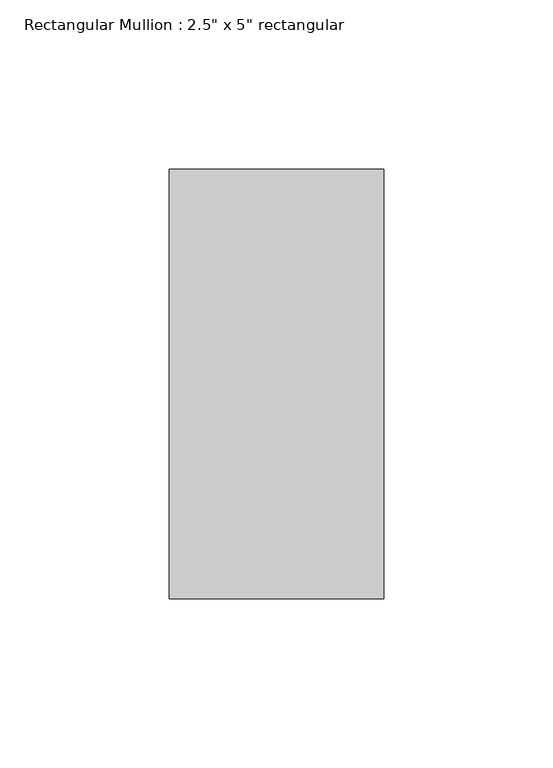
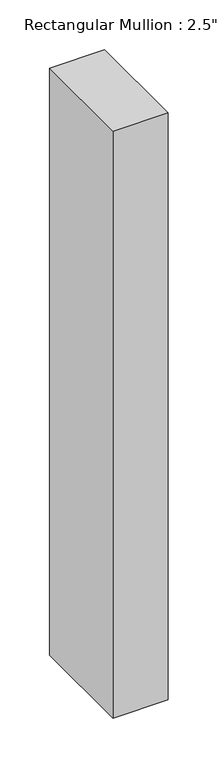
"""IFC4 building model written with IfcOpenShell, lengths in millimetres: member geometry."""

from ifc_helpers import new_model, si_unit, frame, origin, place, context, project, spatial, polyline, outline, extrude, source, transform, mapped, element, save


def member_abeaf8ac(model_context):
    return source(origin(), model_context, "Body", "SweptSolid", [
        extrude(outline(polyline([(31.75, 63.5), (31.75, -63.5), (-31.75, -63.5), (-31.75, 63.5), (31.75, 63.5)])), frame((0.0, 0.0, -717.55), z_axis=(0.0, 0.0, 1.0), x_axis=(1.0, 0.0, 0.0)), (0.0, 0.0, 1.0), 717.55),
    ])


if __name__ == "__main__":
    model = new_model("IFC4")
    model_context = context("Model", 3, world=origin())
    ifc_project = project(units=[si_unit("LENGTHUNIT", "METRE", prefix="MILLI")], contexts=[model_context])
    site = spatial("IfcSite", under=ifc_project)
    building = spatial("IfcBuilding", under=site)
    placement = place(None, origin())
    member_shape = member_abeaf8ac(model_context)
    element("IfcMember", 1, ObjectType="Rectangular Mullion : 2.5\" x 5\" rectangular", at=placement, inside=building, context=model_context, shape_type="MappedRepresentation", body=[
        mapped(member_shape, transform((0.0, 0.0, 0.0), x_axis=(1.0, 0.0, 0.0), y_axis=(0.0, 1.0, 0.0), z_axis=(0.0, 0.0, 1.0))),
    ])
    save(model, "model.ifc")

# Revit data of these elements
# Type "Rectangular Mullion : 2.5\" x 5\" rectangular"
#   built-in parameter 1007304 = 0.416667 (stored number, unit not read)
#   built-in parameter 1007301 = 0.104167 (stored number, unit not read)
#   built-in parameter 1007300 = 0.104167 (stored number, unit not read)
# Element 1 (IfcMember, "Rectangular Mullion : 2.5\" x 5\" rectangular")
#   Materials on its faces: "Door - Frame"
# Materials
#   "Door - Frame": colour RGB 118 70 51, transparency 0, Cost = 0
